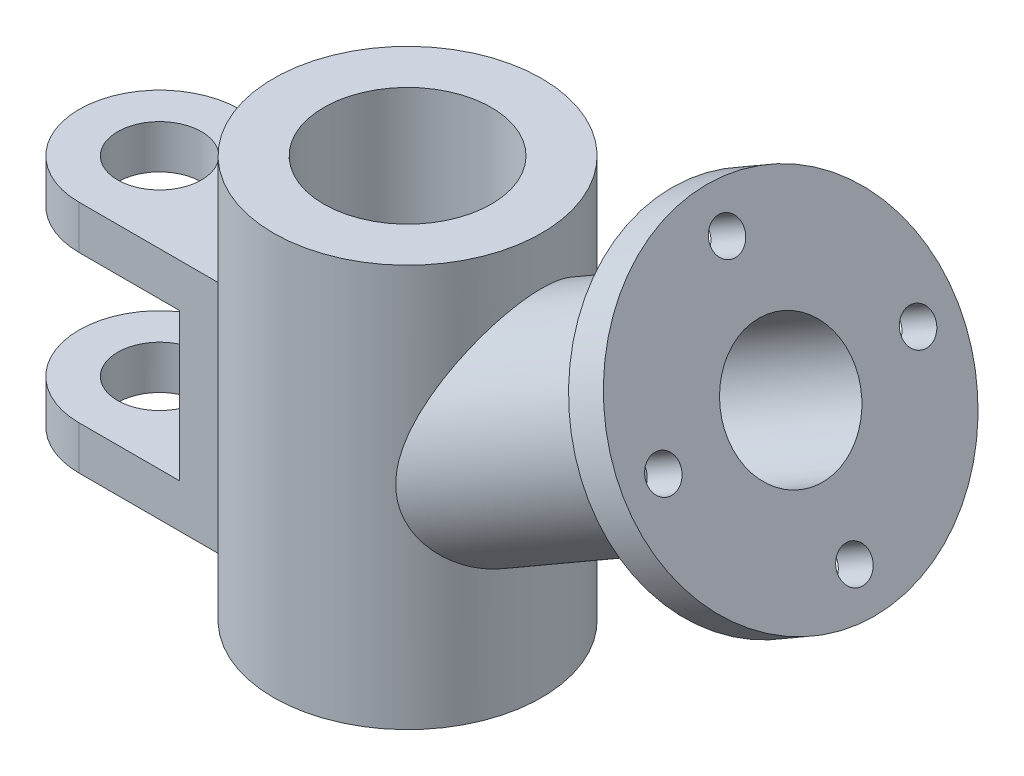
ISO-10303-21;
HEADER;
FILE_DESCRIPTION(('STEP AP214'),'2;1');
FILE_NAME('part.step','',(''),(''),'','','');
FILE_SCHEMA(('AUTOMOTIVE_DESIGN { 1 0 10303 214 1 1 1 1 }'));
ENDSEC;
DATA;
#1=APPLICATION_CONTEXT('core data for automotive mechanical design processes');
#2=APPLICATION_PROTOCOL_DEFINITION('international standard','automotive_design',2000,#1);
#3=PRODUCT_CONTEXT('',#1,'mechanical');
#4=PRODUCT('Part','Part','',(#3));
#5=PRODUCT_RELATED_PRODUCT_CATEGORY('part','',(#4));
#6=PRODUCT_DEFINITION_FORMATION('','',#4);
#7=PRODUCT_DEFINITION_CONTEXT('part definition',#1,'design');
#8=PRODUCT_DEFINITION('design','',#6,#7);
#9=PRODUCT_DEFINITION_SHAPE('','',#8);
#10=(LENGTH_UNIT() NAMED_UNIT(*) SI_UNIT(.MILLI.,.METRE.));
#11=(NAMED_UNIT(*) PLANE_ANGLE_UNIT() SI_UNIT($,.RADIAN.));
#12=(NAMED_UNIT(*) SI_UNIT($,.STERADIAN.) SOLID_ANGLE_UNIT());
#13=UNCERTAINTY_MEASURE_WITH_UNIT(LENGTH_MEASURE(1.E-05),#10,'distance_accuracy_value','');
#14=(GEOMETRIC_REPRESENTATION_CONTEXT(3) GLOBAL_UNCERTAINTY_ASSIGNED_CONTEXT((#13)) GLOBAL_UNIT_ASSIGNED_CONTEXT((#10,
#11,#12)) REPRESENTATION_CONTEXT('',''));
#15=CARTESIAN_POINT('',(0.,0.,0.));
#16=DIRECTION('',(0.,0.,1.));
#17=DIRECTION('',(1.,0.,0.));
#18=AXIS2_PLACEMENT_3D('',#15,#16,#17);
#19=CARTESIAN_POINT('',(-3.7,0.65,0.));
#20=DIRECTION('',(0.,1.,0.));
#21=DIRECTION('',(0.,0.,1.));
#22=AXIS2_PLACEMENT_3D('',#19,#20,#21);
#23=CYLINDRICAL_SURFACE('',#22,1.2);
#24=CARTESIAN_POINT('',(-3.7,3.5,0.));
#25=DIRECTION('',(0.,1.,0.));
#26=DIRECTION('',(0.,0.,1.));
#27=AXIS2_PLACEMENT_3D('',#24,#25,#26);
#28=CIRCLE('',#27,1.2);
#29=CARTESIAN_POINT('',(-3.7,3.5,1.2));
#30=VERTEX_POINT('',#29);
#31=CARTESIAN_POINT('',(-3.7,3.5,-1.2));
#32=VERTEX_POINT('',#31);
#33=EDGE_CURVE('E138',#30,#32,#28,.F.);
#34=ORIENTED_EDGE('',*,*,#33,.F.);
#35=DIRECTION('',(0.,1.,0.));
#36=VECTOR('',#35,1.);
#37=CARTESIAN_POINT('',(-3.7,0.65,1.2));
#38=LINE('',#37,#36);
#39=CARTESIAN_POINT('',(-3.7,4.15,1.2));
#40=VERTEX_POINT('',#39);
#41=EDGE_CURVE('E161',#30,#40,#38,.T.);
#42=ORIENTED_EDGE('',*,*,#41,.T.);
#43=CARTESIAN_POINT('',(-3.7,4.15,0.));
#44=DIRECTION('',(0.,1.,0.));
#45=DIRECTION('',(0.,0.,1.));
#46=AXIS2_PLACEMENT_3D('',#43,#44,#45);
#47=CIRCLE('',#46,1.2);
#48=CARTESIAN_POINT('',(-3.7,4.15,-1.2));
#49=VERTEX_POINT('',#48);
#50=EDGE_CURVE('E149',#49,#40,#47,.T.);
#51=ORIENTED_EDGE('',*,*,#50,.F.);
#52=DIRECTION('',(0.,1.,0.));
#53=VECTOR('',#52,1.);
#54=CARTESIAN_POINT('',(-3.7,0.65,-1.2));
#55=LINE('',#54,#53);
#56=EDGE_CURVE('E168',#32,#49,#55,.T.);
#57=ORIENTED_EDGE('',*,*,#56,.F.);
#58=EDGE_LOOP('',(#34,#42,#51,#57));
#59=FACE_BOUND('',#58,.T.);
#60=ADVANCED_FACE('F37',(#59),#23,.T.);
#61=CARTESIAN_POINT('',(-3.7,0.65,0.));
#62=DIRECTION('',(0.,1.,0.));
#63=DIRECTION('',(0.,0.,1.));
#64=AXIS2_PLACEMENT_3D('',#61,#62,#63);
#65=CYLINDRICAL_SURFACE('',#64,0.625);
#66=CARTESIAN_POINT('',(-3.7,3.5,0.));
#67=DIRECTION('',(0.,1.,0.));
#68=DIRECTION('',(0.,0.,1.));
#69=AXIS2_PLACEMENT_3D('',#66,#67,#68);
#70=CIRCLE('',#69,0.625);
#71=CARTESIAN_POINT('',(-3.7,3.5,0.625));
#72=VERTEX_POINT('',#71);
#73=EDGE_CURVE('E44',#72,#72,#70,.F.);
#74=ORIENTED_EDGE('',*,*,#73,.T.);
#75=EDGE_LOOP('',(#74));
#76=FACE_BOUND('',#75,.T.);
#77=CARTESIAN_POINT('',(-3.7,4.15,0.));
#78=DIRECTION('',(0.,1.,0.));
#79=DIRECTION('',(0.,0.,1.));
#80=AXIS2_PLACEMENT_3D('',#77,#78,#79);
#81=CIRCLE('',#80,0.625);
#82=CARTESIAN_POINT('',(-3.7,4.15,0.625));
#83=VERTEX_POINT('',#82);
#84=EDGE_CURVE('E144',#83,#83,#81,.T.);
#85=ORIENTED_EDGE('',*,*,#84,.T.);
#86=EDGE_LOOP('',(#85));
#87=FACE_BOUND('',#86,.T.);
#88=ADVANCED_FACE('F207',(#76,#87),#65,.F.);
#89=CARTESIAN_POINT('',(0.,6.,0.));
#90=DIRECTION('',(0.,-1.,0.));
#91=DIRECTION('',(0.,0.,-1.));
#92=AXIS2_PLACEMENT_3D('',#89,#90,#91);
#93=CYLINDRICAL_SURFACE('',#92,2.);
#94=CARTESIAN_POINT('',(2.,5.28675134594813,0.));
#95=CARTESIAN_POINT('',(1.9999970486525,5.28674553568537,-0.0509645549548926));
#96=CARTESIAN_POINT('',(1.99803036507296,5.28258531444875,-0.101968074915427));
#97=CARTESIAN_POINT('',(1.99037092425183,5.26634323343092,-0.202425088211594));
#98=CARTESIAN_POINT('',(1.98467255223197,5.25424943657451,-0.251876127969954));
#99=CARTESIAN_POINT('',(1.96845268767769,5.21968619808088,-0.358794338921624));
#100=CARTESIAN_POINT('',(1.95713760119165,5.195501316032,-0.415581233530213));
#101=CARTESIAN_POINT('',(1.93093069375908,5.13907333325674,-0.524059647410448));
#102=CARTESIAN_POINT('',(1.91603305556804,5.10681712305062,-0.575742684638304));
#103=CARTESIAN_POINT('',(1.87551765385294,5.01824597695864,-0.698951661092725));
#104=CARTESIAN_POINT('',(1.84830951140444,4.95805490178913,-0.767139974964058));
#105=CARTESIAN_POINT('',(1.7909867316854,4.8285693881339,-0.892836810800664));
#106=CARTESIAN_POINT('',(1.76086375165627,4.75924860140653,-0.950313212267064));
#107=CARTESIAN_POINT('',(1.70535745654534,4.62776578435047,-1.04604468652679));
#108=CARTESIAN_POINT('',(1.68013462820626,4.56667024504012,-1.08588649630983));
#109=CARTESIAN_POINT('',(1.62986640225519,4.44105499584961,-1.15997484965928));
#110=CARTESIAN_POINT('',(1.60482115283824,4.37653273775444,-1.19421714983622));
#111=CARTESIAN_POINT('',(1.55573541972518,4.24458477197344,-1.25749289608485));
#112=CARTESIAN_POINT('',(1.53169539806281,4.17715775746073,-1.28652396666901));
#113=CARTESIAN_POINT('',(1.48557417432718,4.03974300659564,-1.33951570213413));
#114=CARTESIAN_POINT('',(1.46349179029028,3.96975685193415,-1.3634794387979));
#115=CARTESIAN_POINT('',(1.41737118784856,3.80982531233715,-1.41153033550627));
#116=CARTESIAN_POINT('',(1.39418361541946,3.71919784518041,-1.43420363642414));
#117=CARTESIAN_POINT('',(1.35581738360888,3.53454566238734,-1.47053291818328));
#118=CARTESIAN_POINT('',(1.3406189505389,3.44052995573783,-1.48421118366653));
#119=CARTESIAN_POINT('',(1.32526567903617,3.27709274870488,-1.49791385075284));
#120=CARTESIAN_POINT('',(1.32207565854465,3.20821891129919,-1.50070229442481));
#121=CARTESIAN_POINT('',(1.32401342684527,3.07068145547059,-1.49899977723801));
#122=CARTESIAN_POINT('',(1.32912553603763,3.0020176855799,-1.49452253853183));
#123=CARTESIAN_POINT('',(1.34876732528906,2.86641719439632,-1.47682225044538));
#124=CARTESIAN_POINT('',(1.3633893615177,2.79950417591694,-1.46351340644034));
#125=CARTESIAN_POINT('',(1.40117326229666,2.67083315424934,-1.42736768376759));
#126=CARTESIAN_POINT('',(1.42433998211984,2.60907810644702,-1.40452538701438));
#127=CARTESIAN_POINT('',(1.47309929261382,2.49984301956458,-1.3531675444883));
#128=CARTESIAN_POINT('',(1.4980229287275,2.45154406885291,-1.32572324583763));
#129=CARTESIAN_POINT('',(1.55008786188708,2.36053090509224,-1.26445447180689));
#130=CARTESIAN_POINT('',(1.57723009683264,2.31781907401334,-1.23062729011099));
#131=CARTESIAN_POINT('',(1.6362694232045,2.23143378908336,-1.15127823856732));
#132=CARTESIAN_POINT('',(1.66822410068182,2.18872669231969,-1.10474952104184));
#133=CARTESIAN_POINT('',(1.73021780268166,2.11046463930542,-1.00489325473654));
#134=CARTESIAN_POINT('',(1.7602556711338,2.07491397192563,-0.951561660059982));
#135=CARTESIAN_POINT('',(1.8215574324917,2.00511658459749,-0.829094013256131));
#136=CARTESIAN_POINT('',(1.85210385038894,1.97220471861288,-0.758829269900914));
#137=CARTESIAN_POINT('',(1.90571090628462,1.91599178606554,-0.611874293037778));
#138=CARTESIAN_POINT('',(1.92877005697721,1.89269262876782,-0.535182786689392));
#139=CARTESIAN_POINT('',(1.96612928486342,1.85547486260921,-0.375729769907822));
#140=CARTESIAN_POINT('',(1.98023968653309,1.84175879794579,-0.292875926358499));
#141=CARTESIAN_POINT('',(1.99787194717028,1.82467517260186,-0.125009022886388));
#142=CARTESIAN_POINT('',(2.0013960858517,1.82130538388436,-0.0399964318192956));
#143=CARTESIAN_POINT('',(1.99767178786206,1.82489112866947,0.126401053537316));
#144=CARTESIAN_POINT('',(1.99081819833639,1.83146819713097,0.207803514204965));
#145=CARTESIAN_POINT('',(1.96754322783607,1.85416242103331,0.367848133815773));
#146=CARTESIAN_POINT('',(1.9511225356101,1.87027888972115,0.446490491030453));
#147=CARTESIAN_POINT('',(1.90980367359583,1.91193169591238,0.599094917937578));
#148=CARTESIAN_POINT('',(1.88488577831092,1.93748996331462,0.673045618295913));
#149=CARTESIAN_POINT('',(1.82830377070922,1.99793792859396,0.814308871040709));
#150=CARTESIAN_POINT('',(1.79663459209368,2.03283463927503,0.881616382441848));
#151=CARTESIAN_POINT('',(1.72755963362521,2.11362673862452,1.01048900698373));
#152=CARTESIAN_POINT('',(1.68997619906204,2.15990332800566,1.07172066544373));
#153=CARTESIAN_POINT('',(1.6136025499884,2.26308586171886,1.18357698326777));
#154=CARTESIAN_POINT('',(1.57481371861604,2.3199799728611,1.23421331909035));
#155=CARTESIAN_POINT('',(1.50996145383683,2.4294114009334,1.31222586871969));
#156=CARTESIAN_POINT('',(1.48311287682947,2.47958507915393,1.34226029031302));
#157=CARTESIAN_POINT('',(1.43403484798806,2.58582820557518,1.39457166425866));
#158=CARTESIAN_POINT('',(1.41179654291347,2.64188603634136,1.41686354153033));
#159=CARTESIAN_POINT('',(1.37412739986106,2.75901498960152,1.45343747366988));
#160=CARTESIAN_POINT('',(1.35872528529978,2.82010600995811,1.46768579904074));
#161=CARTESIAN_POINT('',(1.33602066041981,2.94505045755975,1.48838326101344));
#162=CARTESIAN_POINT('',(1.32872485917987,3.00890612758975,1.49482593777565));
#163=CARTESIAN_POINT('',(1.32090236801746,3.15447738653167,1.50175223890729));
#164=CARTESIAN_POINT('',(1.32271103592767,3.23639731724767,1.50017854643198));
#165=CARTESIAN_POINT('',(1.33580137367746,3.39891425648451,1.48851876488665));
#166=CARTESIAN_POINT('',(1.34711435679016,3.47950599305465,1.47840453728718));
#167=CARTESIAN_POINT('',(1.37422073426935,3.62717221607955,1.45320652203402));
#168=CARTESIAN_POINT('',(1.38917140172567,3.69456688661104,1.43901031981333));
#169=CARTESIAN_POINT('',(1.4224713427755,3.82742285900561,1.40610216953895));
#170=CARTESIAN_POINT('',(1.44082329660041,3.89288258862779,1.3873866566974));
#171=CARTESIAN_POINT('',(1.47986276585991,4.02185197422553,1.34566894680336));
#172=CARTESIAN_POINT('',(1.50055502122334,4.08535732882995,1.32265798640131));
#173=CARTESIAN_POINT('',(1.54339714295202,4.21013132612929,1.27240563982987));
#174=CARTESIAN_POINT('',(1.56554640368221,4.27140088192046,1.24516600507478));
#175=CARTESIAN_POINT('',(1.60805791263721,4.38466557044923,1.18963445102772));
#176=CARTESIAN_POINT('',(1.62833707302591,4.43692322817819,1.16181417124925));
#177=CARTESIAN_POINT('',(1.66906630346155,4.53923869329852,1.10250271783841));
#178=CARTESIAN_POINT('',(1.689516337527,4.58929695059075,1.0710122998146));
#179=CARTESIAN_POINT('',(1.73008318094181,4.68665211306674,1.00415977583565));
#180=CARTESIAN_POINT('',(1.7502008577014,4.73395746917606,0.96881059430578));
#181=CARTESIAN_POINT('',(1.78966516512206,4.82533331714667,0.893808138305228));
#182=CARTESIAN_POINT('',(1.80901237163407,4.86940624648568,0.854158164049344));
#183=CARTESIAN_POINT('',(1.84806600077724,4.95730774131388,0.766272620041581));
#184=CARTESIAN_POINT('',(1.86764400675991,5.0007467728831,0.717583720445762));
#185=CARTESIAN_POINT('',(1.904180363692,5.08103454011871,0.61408475785194));
#186=CARTESIAN_POINT('',(1.92114051683689,5.11788781236879,0.559278951076864));
#187=CARTESIAN_POINT('',(1.94844910343736,5.17684036449463,0.453829768030057));
#188=CARTESIAN_POINT('',(1.95943689871934,5.2003977446446,0.404177738052494));
#189=CARTESIAN_POINT('',(1.97785973227975,5.23975954934716,0.301297519571608));
#190=CARTESIAN_POINT('',(1.98530333001162,5.25558265512881,0.248078304654108));
#191=CARTESIAN_POINT('',(1.99368655715187,5.27337683667634,0.161978994939816));
#192=CARTESIAN_POINT('',(1.99604359010548,5.2783718790058,0.129841001902964));
#193=CARTESIAN_POINT('',(1.99920135148534,5.28506119569592,0.0651406813479076));
#194=CARTESIAN_POINT('',(2.00000188660314,5.28675506006852,0.0325783016287044));
#195=CARTESIAN_POINT('',(2.,5.28675134594813,0.));
#196=B_SPLINE_CURVE_WITH_KNOTS('',3,(#94,#95,#96,#97,#98,#99,#100,#101,#102,#103,#104,#105,#106,
#107,#108,#109,#110,#111,#112,#113,#114,#115,#116,#117,#118,#119,#120,#121,#122,#123,#124,#125,
#126,#127,#128,#129,#130,#131,#132,#133,#134,#135,#136,#137,#138,#139,#140,#141,#142,#143,#144,
#145,#146,#147,#148,#149,#150,#151,#152,#153,#154,#155,#156,#157,#158,#159,#160,#161,#162,#163,
#164,#165,#166,#167,#168,#169,#170,#171,#172,#173,#174,#175,#176,#177,#178,#179,#180,#181,#182,
#183,#184,#185,#186,#187,#188,#189,#190,#191,#192,#193,#194,#195),.UNSPECIFIED.,.T.,.F.,(4,2,2,
2,2,2,2,2,2,2,2,2,2,2,2,2,2,2,2,2,2,2,2,2,2,2,2,2,2,2,2,2,2,2,2,2,2,2,2,2,2,2,2,2,2,2,2,2,2,2,
4),(0.,0.15276354826251,0.305757477570657,0.4929639085865,0.680476397337383,0.963704315388515,
1.24776831048418,1.47899948637416,1.71040508858541,1.94191590835847,2.17328598298484,
2.46145461217104,2.74890660464451,2.95522920350617,3.16116258955364,3.36912638856181,
3.57720853957934,3.75918582207613,3.94124043626816,4.1528050091894,4.36449599840936,
4.61350800514627,4.86256944657616,5.11674752585729,5.3708708648723,5.61556537554982,
5.86024227251474,6.10549107591859,6.35092457089976,6.60608846141651,6.8609696528724,
7.05323202781902,7.2451217039618,7.43781017644694,7.63065800638002,7.87513888882805,
8.12042842035551,8.33157859806514,8.54289587616731,8.75464908036291,8.96631481436553,
9.15391855925452,9.34148374826157,9.52843894448834,9.7152516821129,9.91911693538211,
10.1228412106648,10.2903584771779,10.4574691010694,10.5551087054079,10.6527604352733),.UNSPECIFIED.);
#197=CARTESIAN_POINT('',(2.,5.28675134594813,0.));
#198=VERTEX_POINT('',#197);
#199=EDGE_CURVE('E130',#198,#198,#196,.T.);
#200=ORIENTED_EDGE('',*,*,#199,.T.);
#201=EDGE_LOOP('',(#200));
#202=FACE_BOUND('',#201,.T.);
#203=CARTESIAN_POINT('',(0.,0.,0.));
#204=DIRECTION('',(0.,1.,0.));
#205=DIRECTION('',(0.,0.,1.));
#206=AXIS2_PLACEMENT_3D('',#203,#204,#205);
#207=CIRCLE('',#206,2.);
#208=CARTESIAN_POINT('',(0.,0.,2.));
#209=VERTEX_POINT('',#208);
#210=EDGE_CURVE('E177',#209,#209,#207,.T.);
#211=ORIENTED_EDGE('',*,*,#210,.T.);
#212=EDGE_LOOP('',(#211));
#213=FACE_BOUND('',#212,.T.);
#214=CARTESIAN_POINT('',(0.,6.,0.));
#215=DIRECTION('',(0.,1.,0.));
#216=DIRECTION('',(0.,0.,1.));
#217=AXIS2_PLACEMENT_3D('',#214,#215,#216);
#218=CIRCLE('',#217,2.);
#219=CARTESIAN_POINT('',(0.,6.,2.));
#220=VERTEX_POINT('',#219);
#221=EDGE_CURVE('E176',#220,#220,#218,.T.);
#222=ORIENTED_EDGE('',*,*,#221,.F.);
#223=EDGE_LOOP('',(#222));
#224=FACE_BOUND('',#223,.T.);
#225=CARTESIAN_POINT('',(0.,0.65,0.));
#226=DIRECTION('',(0.,1.,0.));
#227=DIRECTION('',(0.,0.,1.));
#228=AXIS2_PLACEMENT_3D('',#225,#226,#227);
#229=CIRCLE('',#228,2.);
#230=CARTESIAN_POINT('',(-1.6,0.65,-1.2));
#231=VERTEX_POINT('',#230);
#232=CARTESIAN_POINT('',(-1.6,0.65,1.2));
#233=VERTEX_POINT('',#232);
#234=EDGE_CURVE('E12',#231,#233,#229,.T.);
#235=ORIENTED_EDGE('',*,*,#234,.F.);
#236=DIRECTION('',(0.,-1.,0.));
#237=VECTOR('',#236,1.);
#238=CARTESIAN_POINT('',(-1.6,6.,-1.2));
#239=LINE('',#238,#237);
#240=CARTESIAN_POINT('',(-1.6,4.15,-1.2));
#241=VERTEX_POINT('',#240);
#242=EDGE_CURVE('E49',#231,#241,#239,.F.);
#243=ORIENTED_EDGE('',*,*,#242,.T.);
#244=CARTESIAN_POINT('',(0.,4.15,0.));
#245=DIRECTION('',(0.,1.,0.));
#246=DIRECTION('',(0.,0.,1.));
#247=AXIS2_PLACEMENT_3D('',#244,#245,#246);
#248=CIRCLE('',#247,2.);
#249=CARTESIAN_POINT('',(-1.6,4.15,1.2));
#250=VERTEX_POINT('',#249);
#251=EDGE_CURVE('E185',#241,#250,#248,.T.);
#252=ORIENTED_EDGE('',*,*,#251,.T.);
#253=DIRECTION('',(0.,-1.,0.));
#254=VECTOR('',#253,1.);
#255=CARTESIAN_POINT('',(-1.6,6.,1.2));
#256=LINE('',#255,#254);
#257=EDGE_CURVE('E190',#250,#233,#256,.T.);
#258=ORIENTED_EDGE('',*,*,#257,.T.);
#259=EDGE_LOOP('',(#235,#243,#252,#258));
#260=FACE_BOUND('',#259,.T.);
#261=ADVANCED_FACE('F45',(#202,#213,#224,#260),#93,.T.);
#262=CARTESIAN_POINT('',(0.,6.,0.));
#263=DIRECTION('',(0.,1.,0.));
#264=DIRECTION('',(0.,0.,1.));
#265=AXIS2_PLACEMENT_3D('',#262,#263,#264);
#266=PLANE('',#265);
#267=ORIENTED_EDGE('',*,*,#221,.T.);
#268=EDGE_LOOP('',(#267));
#269=FACE_BOUND('',#268,.T.);
#270=CARTESIAN_POINT('',(0.,6.,0.));
#271=DIRECTION('',(0.,1.,0.));
#272=DIRECTION('',(0.,0.,1.));
#273=AXIS2_PLACEMENT_3D('',#270,#271,#272);
#274=CIRCLE('',#273,1.25);
#275=CARTESIAN_POINT('',(0.,6.,1.25));
#276=VERTEX_POINT('',#275);
#277=EDGE_CURVE('E173',#276,#276,#274,.T.);
#278=ORIENTED_EDGE('',*,*,#277,.F.);
#279=EDGE_LOOP('',(#278));
#280=FACE_BOUND('',#279,.T.);
#281=ADVANCED_FACE('F390',(#269,#280),#266,.T.);
#282=CARTESIAN_POINT('',(0.,0.,0.));
#283=DIRECTION('',(0.,1.,0.));
#284=DIRECTION('',(0.,0.,1.));
#285=AXIS2_PLACEMENT_3D('',#282,#283,#284);
#286=PLANE('',#285);
#287=ORIENTED_EDGE('',*,*,#210,.F.);
#288=EDGE_LOOP('',(#287));
#289=FACE_BOUND('',#288,.T.);
#290=CARTESIAN_POINT('',(0.,0.,0.));
#291=DIRECTION('',(0.,1.,0.));
#292=DIRECTION('',(0.,0.,1.));
#293=AXIS2_PLACEMENT_3D('',#290,#291,#292);
#294=CIRCLE('',#293,1.25);
#295=CARTESIAN_POINT('',(0.,0.,1.25));
#296=VERTEX_POINT('',#295);
#297=EDGE_CURVE('E166',#296,#296,#294,.T.);
#298=ORIENTED_EDGE('',*,*,#297,.T.);
#299=EDGE_LOOP('',(#298));
#300=FACE_BOUND('',#299,.T.);
#301=ADVANCED_FACE('F252',(#289,#300),#286,.F.);
#302=CARTESIAN_POINT('',(0.,6.,0.));
#303=DIRECTION('',(0.,-1.,0.));
#304=DIRECTION('',(0.,0.,-1.));
#305=AXIS2_PLACEMENT_3D('',#302,#303,#304);
#306=CYLINDRICAL_SURFACE('',#305,1.25);
#307=CARTESIAN_POINT('',(1.25,4.21865334794732,0.));
#308=CARTESIAN_POINT('',(1.24999813614527,4.21864970328222,0.0321026990287067));
#309=CARTESIAN_POINT('',(1.24874910116528,4.21603274633786,0.0642414788663816));
#310=CARTESIAN_POINT('',(1.24388323854935,4.2058141021631,0.127550186545698));
#311=CARTESIAN_POINT('',(1.24026178878809,4.19820268428277,0.158718098435612));
#312=CARTESIAN_POINT('',(1.22995121638852,4.17644874622317,0.226112293741986));
#313=CARTESIAN_POINT('',(1.22275692816389,4.16122578138426,0.261909514552392));
#314=CARTESIAN_POINT('',(1.20609104993659,4.12571330757059,0.330287681274534));
#315=CARTESIAN_POINT('',(1.19661595820644,4.10541600607837,0.36286357190049));
#316=CARTESIAN_POINT('',(1.17081220210405,4.04963137184636,0.44060789765104));
#317=CARTESIAN_POINT('',(1.15346152015805,4.01169379212786,0.483661057654697));
#318=CARTESIAN_POINT('',(1.11687776017897,3.93009437997939,0.563028763773868));
#319=CARTESIAN_POINT('',(1.09763924768612,3.88641589107644,0.599322929048331));
#320=CARTESIAN_POINT('',(1.06202138702507,3.80328761309725,0.660008718693008));
#321=CARTESIAN_POINT('',(1.04574846626571,3.76448547529165,0.685367503879216));
#322=CARTESIAN_POINT('',(1.01328078247239,3.68470717725178,0.73251773677677));
#323=CARTESIAN_POINT('',(0.997086089141574,3.64372936861845,0.754306427024871));
#324=CARTESIAN_POINT('',(0.96530170805266,3.55993319466213,0.794575147664763));
#325=CARTESIAN_POINT('',(0.949712312840895,3.51711395992198,0.813053593398418));
#326=CARTESIAN_POINT('',(0.919747236941378,3.42985128837338,0.846802122620772));
#327=CARTESIAN_POINT('',(0.905370820003192,3.38540886062635,0.862074160828975));
#328=CARTESIAN_POINT('',(0.875416784742906,3.28435933544799,0.892580979692902));
#329=CARTESIAN_POINT('',(0.860345772020769,3.22733996310972,0.906970167297517));
#330=CARTESIAN_POINT('',(0.8351863624843,3.11113441698942,0.93019361500459));
#331=CARTESIAN_POINT('',(0.825086038946662,3.0519537994329,0.939041185782719));
#332=CARTESIAN_POINT('',(0.814544566679323,2.94920919789628,0.948183324565382));
#333=CARTESIAN_POINT('',(0.812167597853762,2.90601707007576,0.950199871613304));
#334=CARTESIAN_POINT('',(0.812675545600198,2.81968887356437,0.949769797426733));
#335=CARTESIAN_POINT('',(0.815550126862748,2.77655286159755,0.947331942673071));
#336=CARTESIAN_POINT('',(0.82734512093803,2.69124838948537,0.93704997913504));
#337=CARTESIAN_POINT('',(0.836328630735141,2.649094823313,0.929149433690343));
#338=CARTESIAN_POINT('',(0.859864631634575,2.56797914574299,0.90740397109388));
#339=CARTESIAN_POINT('',(0.874420070179208,2.52901873672928,0.893555907346669));
#340=CARTESIAN_POINT('',(0.905111669361618,2.46033806665069,0.862370457122187));
#341=CARTESIAN_POINT('',(0.920782355246301,2.43007758269728,0.845739171229618));
#342=CARTESIAN_POINT('',(0.953614681067882,2.37299267998655,0.808538843689019));
#343=CARTESIAN_POINT('',(0.970776995531826,2.3461698294662,0.78796801543309));
#344=CARTESIAN_POINT('',(1.00829540200622,2.29171534591807,0.739544311274648));
#345=CARTESIAN_POINT('',(1.02870685844176,2.26469464124826,0.711049139016081));
#346=CARTESIAN_POINT('',(1.06845670494612,2.215049199112,0.649798021166723));
#347=CARTESIAN_POINT('',(1.08779443421615,2.19242714772653,0.61703949236814));
#348=CARTESIAN_POINT('',(1.12768984115862,2.14757049962821,0.541270698358137));
#349=CARTESIAN_POINT('',(1.14778891732761,2.1262148780489,0.497492467310776));
#350=CARTESIAN_POINT('',(1.18334617794659,2.08948842484067,0.405729083119038));
#351=CARTESIAN_POINT('',(1.19880327000102,2.07411900168825,0.357742943157027));
#352=CARTESIAN_POINT('',(1.22429963303666,2.04915051114397,0.257540600515593));
#353=CARTESIAN_POINT('',(1.23419394696004,2.03970515099553,0.205248681744495));
#354=CARTESIAN_POINT('',(1.24721384243214,2.02733104087638,0.0990790745609366));
#355=CARTESIAN_POINT('',(1.25034104142277,2.02440073370576,0.0452017682010726));
#356=CARTESIAN_POINT('',(1.2496143115555,2.02508596093283,-0.0602937224010105));
#357=CARTESIAN_POINT('',(1.24603531526447,2.02844370225563,-0.111915856706425));
#358=CARTESIAN_POINT('',(1.232683544034,2.04114977187746,-0.213588085827169));
#359=CARTESIAN_POINT('',(1.22291128000496,2.05049760602761,-0.263638309958985));
#360=CARTESIAN_POINT('',(1.19785923536017,2.07505707692805,-0.36075748893584));
#361=CARTESIAN_POINT('',(1.18258597468951,2.09026177342694,-0.407829895855065));
#362=CARTESIAN_POINT('',(1.14756162561547,2.12646188721477,-0.497936167775832));
#363=CARTESIAN_POINT('',(1.12780755766145,2.14746115967683,-0.540967318464282));
#364=CARTESIAN_POINT('',(1.08433851370691,2.19628936935301,-0.623684272381126));
#365=CARTESIAN_POINT('',(1.060492136477,2.22436786610046,-0.663153998685726));
#366=CARTESIAN_POINT('',(1.01159163893849,2.28712426611613,-0.735584303583659));
#367=CARTESIAN_POINT('',(0.986538488008199,2.32179693630893,-0.768550001731208));
#368=CARTESIAN_POINT('',(0.943955310189886,2.38895120001299,-0.819930890727398));
#369=CARTESIAN_POINT('',(0.926057832556045,2.41997749096286,-0.839940750394299));
#370=CARTESIAN_POINT('',(0.892938000205868,2.48594213279277,-0.875067752063272));
#371=CARTESIAN_POINT('',(0.87771030035859,2.52087243235558,-0.890194722350042));
#372=CARTESIAN_POINT('',(0.851464812509628,2.59429182913414,-0.915339413392153));
#373=CARTESIAN_POINT('',(0.840472512843486,2.63280079316032,-0.925326318720514));
#374=CARTESIAN_POINT('',(0.823830943115782,2.71190260756079,-0.94017468856974));
#375=CARTESIAN_POINT('',(0.818184786166763,2.7524966576163,-0.945033166944918));
#376=CARTESIAN_POINT('',(0.811522963885866,2.84235194078356,-0.950765885076619));
#377=CARTESIAN_POINT('',(0.811635383410467,2.89174865366688,-0.950669468190259));
#378=CARTESIAN_POINT('',(0.81775058885594,2.98992103952507,-0.945405769130707));
#379=CARTESIAN_POINT('',(0.823770583414345,3.03869447638518,-0.940223672479935));
#380=CARTESIAN_POINT('',(0.838838295322252,3.1283070211887,-0.926788438465457));
#381=CARTESIAN_POINT('',(0.847360700322198,3.16932056492162,-0.919050919896149));
#382=CARTESIAN_POINT('',(0.866607232338006,3.25025099593715,-0.900925435149091));
#383=CARTESIAN_POINT('',(0.877333095701186,3.29016699004074,-0.890535377166827));
#384=CARTESIAN_POINT('',(0.900345417394656,3.36895537952556,-0.86726413042715));
#385=CARTESIAN_POINT('',(0.912637111777876,3.40782371742477,-0.854374504030582));
#386=CARTESIAN_POINT('',(0.938238760963884,3.48433031892558,-0.826178531887488));
#387=CARTESIAN_POINT('',(0.951548822612531,3.52196845286277,-0.810871932375353));
#388=CARTESIAN_POINT('',(0.980003250046636,3.59925237596733,-0.77629863425639));
#389=CARTESIAN_POINT('',(0.99520483527315,3.63877350686977,-0.756799389533526));
#390=CARTESIAN_POINT('',(1.02587974134444,3.71604011224703,-0.714668291611172));
#391=CARTESIAN_POINT('',(1.04135320571359,3.75378460765153,-0.692034737618168));
#392=CARTESIAN_POINT('',(1.07203128336141,3.82688867503852,-0.643482398054762));
#393=CARTESIAN_POINT('',(1.08723692135612,3.86226050984017,-0.617582883726999));
#394=CARTESIAN_POINT('',(1.11695931946486,3.93020916190778,-0.562043724284678));
#395=CARTESIAN_POINT('',(1.1314769913262,3.96278972746879,-0.532409231295577));
#396=CARTESIAN_POINT('',(1.15735686405484,4.02012517277403,-0.473205665808765));
#397=CARTESIAN_POINT('',(1.16888106921439,4.0453434929776,-0.444161540350015));
#398=CARTESIAN_POINT('',(1.19043404703174,4.09211118344551,-0.38265898759457));
#399=CARTESIAN_POINT('',(1.20046176467966,4.11365796681372,-0.350198178804163));
#400=CARTESIAN_POINT('',(1.21843869037146,4.15205875918627,-0.281403604004611));
#401=CARTESIAN_POINT('',(1.22635786243426,4.16884515531613,-0.245023279758547));
#402=CARTESIAN_POINT('',(1.23905601272055,4.19567269016587,-0.169385408055287));
#403=CARTESIAN_POINT('',(1.24384793699043,4.20574164138597,-0.130140480000971));
#404=CARTESIAN_POINT('',(1.24781992704368,4.2140806369447,-0.0753111558685922));
#405=CARTESIAN_POINT('',(1.24863484074897,4.21579031802429,-0.0603162501790653));
#406=CARTESIAN_POINT('',(1.24972537085785,4.21807764668261,-0.0302169093872325));
#407=CARTESIAN_POINT('',(1.25000087741583,4.21865506368557,-0.0151124526042312));
#408=CARTESIAN_POINT('',(1.25,4.21865334794732,0.));
#409=B_SPLINE_CURVE_WITH_KNOTS('',3,(#307,#308,#309,#310,#311,#312,#313,#314,#315,#316,#317,
#318,#319,#320,#321,#322,#323,#324,#325,#326,#327,#328,#329,#330,#331,#332,#333,#334,#335,#336,
#337,#338,#339,#340,#341,#342,#343,#344,#345,#346,#347,#348,#349,#350,#351,#352,#353,#354,#355,
#356,#357,#358,#359,#360,#361,#362,#363,#364,#365,#366,#367,#368,#369,#370,#371,#372,#373,#374,
#375,#376,#377,#378,#379,#380,#381,#382,#383,#384,#385,#386,#387,#388,#389,#390,#391,#392,#393,
#394,#395,#396,#397,#398,#399,#400,#401,#402,#403,#404,#405,#406,#407,#408),.UNSPECIFIED.,.T.,
.F.,(4,2,2,2,2,2,2,2,2,2,2,2,2,2,2,2,2,2,2,2,2,2,2,2,2,2,2,2,2,2,2,2,2,2,2,2,2,2,2,2,2,2,2,2,2,
2,2,2,2,2,4),(0.,0.0962461091854084,0.192680292531519,0.310696840900612,0.428895749391761,
0.60774366668795,0.78712243985762,0.934312576875,1.0816158698249,1.22898949147428,
1.37627300730675,1.55803396407407,1.73935664916152,1.86884616013595,1.99808110385065,
2.12867156085191,2.25933119334531,2.37266665009142,2.48605362743651,2.61834744281429,
2.75072179273056,2.9080802758821,3.06547576115336,3.22680234120961,3.38809035753427,
3.54291029526456,3.69771746286691,3.85234174895706,4.00706915676485,4.16828767454405,
4.32937878066476,4.45198667616804,4.57434622482995,4.69743103335025,4.82058747139082,
4.96794742962435,5.11573792228422,5.24335937442764,5.3710817819931,5.49924308491356,
5.62741785285046,5.76714120102705,5.90694066760651,6.04595077395733,6.18477118293518,
6.30496154250676,6.42523623890345,6.54714224694145,6.66854033742829,6.71383929044772,
6.75914746724947),.UNSPECIFIED.);
#410=CARTESIAN_POINT('',(1.25,4.21865334794732,0.));
#411=VERTEX_POINT('',#410);
#412=EDGE_CURVE('E458',#411,#411,#409,.T.);
#413=ORIENTED_EDGE('',*,*,#412,.T.);
#414=EDGE_LOOP('',(#413));
#415=FACE_BOUND('',#414,.T.);
#416=ORIENTED_EDGE('',*,*,#277,.T.);
#417=EDGE_LOOP('',(#416));
#418=FACE_BOUND('',#417,.T.);
#419=ORIENTED_EDGE('',*,*,#297,.F.);
#420=EDGE_LOOP('',(#419));
#421=FACE_BOUND('',#420,.T.);
#422=ADVANCED_FACE('F250',(#415,#418,#421),#306,.F.);
#423=CARTESIAN_POINT('',(-3.7,0.65,-1.2));
#424=DIRECTION('',(0.,0.,-1.));
#425=DIRECTION('',(-1.,0.,0.));
#426=AXIS2_PLACEMENT_3D('',#423,#424,#425);
#427=PLANE('',#426);
#428=DIRECTION('',(1.,0.,0.));
#429=VECTOR('',#428,1.);
#430=CARTESIAN_POINT('',(-3.7,3.5,-1.2));
#431=LINE('',#430,#429);
#432=CARTESIAN_POINT('',(-2.2,3.5,-1.2));
#433=VERTEX_POINT('',#432);
#434=EDGE_CURVE('E142',#32,#433,#431,.T.);
#435=ORIENTED_EDGE('',*,*,#434,.F.);
#436=ORIENTED_EDGE('',*,*,#56,.T.);
#437=DIRECTION('',(-1.,0.,0.));
#438=VECTOR('',#437,1.);
#439=CARTESIAN_POINT('',(-3.7,4.15,-1.2));
#440=LINE('',#439,#438);
#441=EDGE_CURVE('E156',#241,#49,#440,.T.);
#442=ORIENTED_EDGE('',*,*,#441,.F.);
#443=ORIENTED_EDGE('',*,*,#242,.F.);
#444=DIRECTION('',(-1.,0.,0.));
#445=VECTOR('',#444,1.);
#446=CARTESIAN_POINT('',(-3.7,0.65,-1.2));
#447=LINE('',#446,#445);
#448=CARTESIAN_POINT('',(-3.7,0.65,-1.2));
#449=VERTEX_POINT('',#448);
#450=EDGE_CURVE('E157',#231,#449,#447,.T.);
#451=ORIENTED_EDGE('',*,*,#450,.T.);
#452=CARTESIAN_POINT('',(-3.7,1.3,-1.2));
#453=VERTEX_POINT('',#452);
#454=EDGE_CURVE('E167',#449,#453,#55,.T.);
#455=ORIENTED_EDGE('',*,*,#454,.T.);
#456=DIRECTION('',(-1.,0.,0.));
#457=VECTOR('',#456,1.);
#458=CARTESIAN_POINT('',(-3.7,1.3,-1.2));
#459=LINE('',#458,#457);
#460=CARTESIAN_POINT('',(-2.2,1.3,-1.2));
#461=VERTEX_POINT('',#460);
#462=EDGE_CURVE('E59',#461,#453,#459,.T.);
#463=ORIENTED_EDGE('',*,*,#462,.F.);
#464=DIRECTION('',(0.,-1.,0.));
#465=VECTOR('',#464,1.);
#466=CARTESIAN_POINT('',(-2.2,0.65,-1.2));
#467=LINE('',#466,#465);
#468=EDGE_CURVE('E117',#433,#461,#467,.T.);
#469=ORIENTED_EDGE('',*,*,#468,.F.);
#470=EDGE_LOOP('',(#435,#436,#442,#443,#451,#455,#463,#469));
#471=FACE_BOUND('',#470,.T.);
#472=ADVANCED_FACE('F232',(#471),#427,.T.);
#473=CARTESIAN_POINT('',(-1.46144263171015,0.65,1.2));
#474=DIRECTION('',(0.,0.,1.));
#475=DIRECTION('',(1.,0.,0.));
#476=AXIS2_PLACEMENT_3D('',#473,#474,#475);
#477=PLANE('',#476);
#478=DIRECTION('',(-1.,0.,0.));
#479=VECTOR('',#478,1.);
#480=CARTESIAN_POINT('',(-4.9,3.5,1.2));
#481=LINE('',#480,#479);
#482=CARTESIAN_POINT('',(-2.2,3.5,1.2));
#483=VERTEX_POINT('',#482);
#484=EDGE_CURVE('E118',#483,#30,#481,.T.);
#485=ORIENTED_EDGE('',*,*,#484,.F.);
#486=DIRECTION('',(0.,1.,0.));
#487=VECTOR('',#486,1.);
#488=CARTESIAN_POINT('',(-2.2,3.5,1.2));
#489=LINE('',#488,#487);
#490=CARTESIAN_POINT('',(-2.2,1.3,1.2));
#491=VERTEX_POINT('',#490);
#492=EDGE_CURVE('E114',#491,#483,#489,.T.);
#493=ORIENTED_EDGE('',*,*,#492,.F.);
#494=DIRECTION('',(1.,0.,0.));
#495=VECTOR('',#494,1.);
#496=CARTESIAN_POINT('',(-4.9,1.3,1.2));
#497=LINE('',#496,#495);
#498=CARTESIAN_POINT('',(-3.7,1.3,1.2));
#499=VERTEX_POINT('',#498);
#500=EDGE_CURVE('E122',#499,#491,#497,.T.);
#501=ORIENTED_EDGE('',*,*,#500,.F.);
#502=CARTESIAN_POINT('',(-3.7,0.65,1.2));
#503=VERTEX_POINT('',#502);
#504=EDGE_CURVE('E172',#503,#499,#38,.T.);
#505=ORIENTED_EDGE('',*,*,#504,.F.);
#506=DIRECTION('',(1.,0.,0.));
#507=VECTOR('',#506,1.);
#508=CARTESIAN_POINT('',(-1.46144263171015,0.65,1.2));
#509=LINE('',#508,#507);
#510=EDGE_CURVE('E154',#503,#233,#509,.T.);
#511=ORIENTED_EDGE('',*,*,#510,.T.);
#512=ORIENTED_EDGE('',*,*,#257,.F.);
#513=DIRECTION('',(1.,0.,0.));
#514=VECTOR('',#513,1.);
#515=CARTESIAN_POINT('',(-1.46144263171015,4.15,1.2));
#516=LINE('',#515,#514);
#517=EDGE_CURVE('E67',#40,#250,#516,.T.);
#518=ORIENTED_EDGE('',*,*,#517,.F.);
#519=ORIENTED_EDGE('',*,*,#41,.F.);
#520=EDGE_LOOP('',(#485,#493,#501,#505,#511,#512,#518,#519));
#521=FACE_BOUND('',#520,.T.);
#522=ADVANCED_FACE('F129',(#521),#477,.T.);
#523=ORIENTED_EDGE('',*,*,#504,.T.);
#524=CARTESIAN_POINT('',(-3.7,1.3,0.));
#525=DIRECTION('',(0.,-1.,0.));
#526=DIRECTION('',(0.,0.,-1.));
#527=AXIS2_PLACEMENT_3D('',#524,#525,#526);
#528=CIRCLE('',#527,1.2);
#529=EDGE_CURVE('E121',#453,#499,#528,.F.);
#530=ORIENTED_EDGE('',*,*,#529,.F.);
#531=ORIENTED_EDGE('',*,*,#454,.F.);
#532=CARTESIAN_POINT('',(-3.7,0.65,0.));
#533=DIRECTION('',(0.,1.,0.));
#534=DIRECTION('',(0.,0.,1.));
#535=AXIS2_PLACEMENT_3D('',#532,#533,#534);
#536=CIRCLE('',#535,1.2);
#537=EDGE_CURVE('E155',#449,#503,#536,.T.);
#538=ORIENTED_EDGE('',*,*,#537,.T.);
#539=EDGE_LOOP('',(#523,#530,#531,#538));
#540=FACE_BOUND('',#539,.T.);
#541=ADVANCED_FACE('F215',(#540),#23,.T.);
#542=CARTESIAN_POINT('',(-3.7,0.65,0.));
#543=DIRECTION('',(0.,1.,0.));
#544=DIRECTION('',(0.,0.,1.));
#545=AXIS2_PLACEMENT_3D('',#542,#543,#544);
#546=PLANE('',#545);
#547=CARTESIAN_POINT('',(-3.7,0.65,0.));
#548=DIRECTION('',(0.,1.,0.));
#549=DIRECTION('',(0.,0.,1.));
#550=AXIS2_PLACEMENT_3D('',#547,#548,#549);
#551=CIRCLE('',#550,0.625);
#552=CARTESIAN_POINT('',(-3.7,0.65,0.625));
#553=VERTEX_POINT('',#552);
#554=EDGE_CURVE('E148',#553,#553,#551,.T.);
#555=ORIENTED_EDGE('',*,*,#554,.T.);
#556=EDGE_LOOP('',(#555));
#557=FACE_BOUND('',#556,.T.);
#558=ORIENTED_EDGE('',*,*,#450,.F.);
#559=ORIENTED_EDGE('',*,*,#234,.T.);
#560=ORIENTED_EDGE('',*,*,#510,.F.);
#561=ORIENTED_EDGE('',*,*,#537,.F.);
#562=EDGE_LOOP('',(#558,#559,#560,#561));
#563=FACE_BOUND('',#562,.T.);
#564=ADVANCED_FACE('F222',(#557,#563),#546,.F.);
#565=CARTESIAN_POINT('',(-3.7,4.15,0.));
#566=DIRECTION('',(0.,1.,0.));
#567=DIRECTION('',(0.,0.,1.));
#568=AXIS2_PLACEMENT_3D('',#565,#566,#567);
#569=PLANE('',#568);
#570=ORIENTED_EDGE('',*,*,#251,.F.);
#571=ORIENTED_EDGE('',*,*,#441,.T.);
#572=ORIENTED_EDGE('',*,*,#50,.T.);
#573=ORIENTED_EDGE('',*,*,#517,.T.);
#574=EDGE_LOOP('',(#570,#571,#572,#573));
#575=FACE_BOUND('',#574,.T.);
#576=ORIENTED_EDGE('',*,*,#84,.F.);
#577=EDGE_LOOP('',(#576));
#578=FACE_BOUND('',#577,.T.);
#579=ADVANCED_FACE('F228',(#575,#578),#569,.T.);
#580=CARTESIAN_POINT('',(-3.7,1.3,0.));
#581=DIRECTION('',(0.,-1.,0.));
#582=DIRECTION('',(0.,0.,-1.));
#583=AXIS2_PLACEMENT_3D('',#580,#581,#582);
#584=CIRCLE('',#583,0.625);
#585=CARTESIAN_POINT('',(-3.7,1.3,-0.625));
#586=VERTEX_POINT('',#585);
#587=EDGE_CURVE('E137',#586,#586,#584,.F.);
#588=ORIENTED_EDGE('',*,*,#587,.T.);
#589=EDGE_LOOP('',(#588));
#590=FACE_BOUND('',#589,.T.);
#591=ORIENTED_EDGE('',*,*,#554,.F.);
#592=EDGE_LOOP('',(#591));
#593=FACE_BOUND('',#592,.T.);
#594=ADVANCED_FACE('F191',(#590,#593),#65,.F.);
#595=CARTESIAN_POINT('',(-4.9,3.5,-2.3));
#596=DIRECTION('',(0.,1.,0.));
#597=DIRECTION('',(0.,0.,1.));
#598=AXIS2_PLACEMENT_3D('',#595,#596,#597);
#599=PLANE('',#598);
#600=ORIENTED_EDGE('',*,*,#434,.T.);
#601=DIRECTION('',(0.,0.,1.));
#602=VECTOR('',#601,1.);
#603=CARTESIAN_POINT('',(-2.2,3.5,-2.3));
#604=LINE('',#603,#602);
#605=EDGE_CURVE('E120',#433,#483,#604,.T.);
#606=ORIENTED_EDGE('',*,*,#605,.T.);
#607=ORIENTED_EDGE('',*,*,#484,.T.);
#608=ORIENTED_EDGE('',*,*,#33,.T.);
#609=EDGE_LOOP('',(#600,#606,#607,#608));
#610=FACE_BOUND('',#609,.T.);
#611=ORIENTED_EDGE('',*,*,#73,.F.);
#612=EDGE_LOOP('',(#611));
#613=FACE_BOUND('',#612,.T.);
#614=ADVANCED_FACE('F197',(#610,#613),#599,.F.);
#615=CARTESIAN_POINT('',(-4.9,1.3,-2.3));
#616=DIRECTION('',(0.,-1.,0.));
#617=DIRECTION('',(0.,0.,-1.));
#618=AXIS2_PLACEMENT_3D('',#615,#616,#617);
#619=PLANE('',#618);
#620=ORIENTED_EDGE('',*,*,#462,.T.);
#621=ORIENTED_EDGE('',*,*,#529,.T.);
#622=ORIENTED_EDGE('',*,*,#500,.T.);
#623=DIRECTION('',(0.,0.,1.));
#624=VECTOR('',#623,1.);
#625=CARTESIAN_POINT('',(-2.2,1.3,-2.3));
#626=LINE('',#625,#624);
#627=EDGE_CURVE('E107',#461,#491,#626,.T.);
#628=ORIENTED_EDGE('',*,*,#627,.F.);
#629=EDGE_LOOP('',(#620,#621,#622,#628));
#630=FACE_BOUND('',#629,.T.);
#631=ORIENTED_EDGE('',*,*,#587,.F.);
#632=EDGE_LOOP('',(#631));
#633=FACE_BOUND('',#632,.T.);
#634=ADVANCED_FACE('F125',(#630,#633),#619,.F.);
#635=CARTESIAN_POINT('',(-2.2,3.5,-2.3));
#636=DIRECTION('',(1.,0.,0.));
#637=DIRECTION('',(0.,1.,0.));
#638=AXIS2_PLACEMENT_3D('',#635,#636,#637);
#639=PLANE('',#638);
#640=ORIENTED_EDGE('',*,*,#468,.T.);
#641=ORIENTED_EDGE('',*,*,#627,.T.);
#642=ORIENTED_EDGE('',*,*,#492,.T.);
#643=ORIENTED_EDGE('',*,*,#605,.F.);
#644=EDGE_LOOP('',(#640,#641,#642,#643));
#645=FACE_BOUND('',#644,.T.);
#646=ADVANCED_FACE('F109',(#645),#639,.F.);
#647=CARTESIAN_POINT('',(0.86602540378444,2.9,0.));
#648=DIRECTION('',(0.866025403784438,0.500000000000001,0.));
#649=DIRECTION('',(-0.500000000000001,0.866025403784438,0.));
#650=AXIS2_PLACEMENT_3D('',#647,#648,#649);
#651=CYLINDRICAL_SURFACE('',#650,1.5);
#652=CARTESIAN_POINT('',(5.19615242270663,5.40000000000001,0.));
#653=DIRECTION('',(0.866025403784438,0.500000000000001,0.));
#654=DIRECTION('',(-0.500000000000001,0.866025403784438,0.));
#655=AXIS2_PLACEMENT_3D('',#652,#653,#654);
#656=CIRCLE('',#655,1.5);
#657=CARTESIAN_POINT('',(4.44615242270663,6.69903810567666,0.));
#658=VERTEX_POINT('',#657);
#659=EDGE_CURVE('E450',#658,#658,#656,.T.);
#660=ORIENTED_EDGE('',*,*,#659,.F.);
#661=EDGE_LOOP('',(#660));
#662=FACE_BOUND('',#661,.T.);
#663=ORIENTED_EDGE('',*,*,#199,.F.);
#664=EDGE_LOOP('',(#663));
#665=FACE_BOUND('',#664,.T.);
#666=ADVANCED_FACE('F201',(#662,#665),#651,.T.);
#667=CARTESIAN_POINT('',(5.7157676649773,5.70000000000001,0.));
#668=DIRECTION('',(0.866025403784438,0.500000000000001,0.));
#669=DIRECTION('',(-0.500000000000001,0.866025403784438,0.));
#670=AXIS2_PLACEMENT_3D('',#667,#668,#669);
#671=PLANE('',#670);
#672=CARTESIAN_POINT('',(5.7157676649773,5.70000000000001,0.));
#673=DIRECTION('',(0.866025403784438,0.500000000000001,0.));
#674=DIRECTION('',(-0.500000000000001,0.866025403784438,0.));
#675=AXIS2_PLACEMENT_3D('',#672,#673,#674);
#676=CIRCLE('',#675,0.95);
#677=CARTESIAN_POINT('',(5.2407676649773,6.52272413359523,0.));
#678=VERTEX_POINT('',#677);
#679=EDGE_CURVE('E470',#678,#678,#676,.T.);
#680=ORIENTED_EDGE('',*,*,#679,.F.);
#681=EDGE_LOOP('',(#680));
#682=FACE_BOUND('',#681,.T.);
#683=CARTESIAN_POINT('',(6.66576754230468,4.05455194528478,-2.45345260654372E-07));
#684=DIRECTION('',(0.866025403784438,0.500000000000001,0.));
#685=DIRECTION('',(-0.500000000000001,0.866025403784438,0.));
#686=AXIS2_PLACEMENT_3D('',#683,#684,#685);
#687=CIRCLE('',#686,0.25);
#688=CARTESIAN_POINT('',(6.54076754230468,4.27105829623089,-2.45345260654372E-07));
#689=VERTEX_POINT('',#688);
#690=EDGE_CURVE('E478',#689,#689,#687,.T.);
#691=ORIENTED_EDGE('',*,*,#690,.F.);
#692=EDGE_LOOP('',(#691));
#693=FACE_BOUND('',#692,.T.);
#694=CARTESIAN_POINT('',(4.76576766497729,7.34544826719044,0.));
#695=DIRECTION('',(0.866025403784438,0.500000000000001,0.));
#696=DIRECTION('',(-0.500000000000001,0.866025403784438,0.));
#697=AXIS2_PLACEMENT_3D('',#694,#695,#696);
#698=CIRCLE('',#697,0.25);
#699=CARTESIAN_POINT('',(4.64076766497729,7.56195461813655,0.));
#700=VERTEX_POINT('',#699);
#701=EDGE_CURVE('E488',#700,#700,#698,.T.);
#702=ORIENTED_EDGE('',*,*,#701,.F.);
#703=EDGE_LOOP('',(#702));
#704=FACE_BOUND('',#703,.T.);
#705=CARTESIAN_POINT('',(5.7157676649773,5.70000000000001,0.));
#706=DIRECTION('',(0.866025403784438,0.500000000000001,0.));
#707=DIRECTION('',(-0.500000000000001,0.866025403784438,0.));
#708=AXIS2_PLACEMENT_3D('',#705,#706,#707);
#709=CIRCLE('',#708,2.5);
#710=CARTESIAN_POINT('',(4.46576766497729,7.86506350946111,0.));
#711=VERTEX_POINT('',#710);
#712=EDGE_CURVE('E449',#711,#711,#709,.T.);
#713=ORIENTED_EDGE('',*,*,#712,.T.);
#714=EDGE_LOOP('',(#713));
#715=FACE_BOUND('',#714,.T.);
#716=CARTESIAN_POINT('',(5.71576754230467,5.70000021247523,-1.90000000000001));
#717=DIRECTION('',(0.866025403784438,0.500000000000001,0.));
#718=DIRECTION('',(-0.500000000000001,0.866025403784438,0.));
#719=AXIS2_PLACEMENT_3D('',#716,#717,#718);
#720=CIRCLE('',#719,0.25);
#721=CARTESIAN_POINT('',(5.59076754230467,5.91650656342134,-1.90000000000001));
#722=VERTEX_POINT('',#721);
#723=EDGE_CURVE('E485',#722,#722,#720,.T.);
#724=ORIENTED_EDGE('',*,*,#723,.F.);
#725=EDGE_LOOP('',(#724));
#726=FACE_BOUND('',#725,.T.);
#727=CARTESIAN_POINT('',(5.7157676649773,5.7,1.89999975465475));
#728=DIRECTION('',(0.866025403784438,0.500000000000001,0.));
#729=DIRECTION('',(-0.500000000000001,0.866025403784438,0.));
#730=AXIS2_PLACEMENT_3D('',#727,#728,#729);
#731=CIRCLE('',#730,0.25);
#732=CARTESIAN_POINT('',(5.5907676649773,5.91650635094611,1.89999975465475));
#733=VERTEX_POINT('',#732);
#734=EDGE_CURVE('E468',#733,#733,#731,.T.);
#735=ORIENTED_EDGE('',*,*,#734,.F.);
#736=EDGE_LOOP('',(#735));
#737=FACE_BOUND('',#736,.T.);
#738=ADVANCED_FACE('F289',(#682,#693,#704,#715,#726,#737),#671,.T.);
#739=CARTESIAN_POINT('',(5.19615242270663,5.40000000000001,0.));
#740=DIRECTION('',(0.866025403784438,0.500000000000001,0.));
#741=DIRECTION('',(-0.500000000000001,0.866025403784438,0.));
#742=AXIS2_PLACEMENT_3D('',#739,#740,#741);
#743=PLANE('',#742);
#744=ORIENTED_EDGE('',*,*,#659,.T.);
#745=EDGE_LOOP('',(#744));
#746=FACE_BOUND('',#745,.T.);
#747=CARTESIAN_POINT('',(5.19615242270663,5.40000000000001,0.));
#748=DIRECTION('',(0.866025403784438,0.500000000000001,0.));
#749=DIRECTION('',(-0.500000000000001,0.866025403784438,0.));
#750=AXIS2_PLACEMENT_3D('',#747,#748,#749);
#751=CIRCLE('',#750,2.5);
#752=CARTESIAN_POINT('',(3.94615242270663,7.56506350946111,0.));
#753=VERTEX_POINT('',#752);
#754=EDGE_CURVE('E491',#753,#753,#751,.T.);
#755=ORIENTED_EDGE('',*,*,#754,.F.);
#756=EDGE_LOOP('',(#755));
#757=FACE_BOUND('',#756,.T.);
#758=CARTESIAN_POINT('',(4.24615242270663,7.04544826719044,0.));
#759=DIRECTION('',(0.866025403784438,0.500000000000001,0.));
#760=DIRECTION('',(-0.500000000000001,0.866025403784438,0.));
#761=AXIS2_PLACEMENT_3D('',#758,#759,#760);
#762=CIRCLE('',#761,0.25);
#763=CARTESIAN_POINT('',(4.12115242270663,7.26195461813655,0.));
#764=VERTEX_POINT('',#763);
#765=EDGE_CURVE('E484',#764,#764,#762,.T.);
#766=ORIENTED_EDGE('',*,*,#765,.T.);
#767=EDGE_LOOP('',(#766));
#768=FACE_BOUND('',#767,.T.);
#769=CARTESIAN_POINT('',(5.19615230003401,5.40000021247523,-1.90000000000001));
#770=DIRECTION('',(0.866025403784438,0.500000000000001,0.));
#771=DIRECTION('',(-0.500000000000001,0.866025403784438,0.));
#772=AXIS2_PLACEMENT_3D('',#769,#770,#771);
#773=CIRCLE('',#772,0.25);
#774=CARTESIAN_POINT('',(5.07115230003401,5.61650656342134,-1.90000000000001));
#775=VERTEX_POINT('',#774);
#776=EDGE_CURVE('E479',#775,#775,#773,.T.);
#777=ORIENTED_EDGE('',*,*,#776,.T.);
#778=EDGE_LOOP('',(#777));
#779=FACE_BOUND('',#778,.T.);
#780=CARTESIAN_POINT('',(6.14615230003402,3.75455194528478,-2.45345260654372E-07));
#781=DIRECTION('',(0.866025403784438,0.500000000000001,0.));
#782=DIRECTION('',(-0.500000000000001,0.866025403784438,0.));
#783=AXIS2_PLACEMENT_3D('',#780,#781,#782);
#784=CIRCLE('',#783,0.25);
#785=CARTESIAN_POINT('',(6.02115230003402,3.97105829623089,-2.45345260654372E-07));
#786=VERTEX_POINT('',#785);
#787=EDGE_CURVE('E471',#786,#786,#784,.T.);
#788=ORIENTED_EDGE('',*,*,#787,.T.);
#789=EDGE_LOOP('',(#788));
#790=FACE_BOUND('',#789,.T.);
#791=CARTESIAN_POINT('',(5.19615242270664,5.4,1.89999975465475));
#792=DIRECTION('',(0.866025403784438,0.500000000000001,0.));
#793=DIRECTION('',(-0.500000000000001,0.866025403784438,0.));
#794=AXIS2_PLACEMENT_3D('',#791,#792,#793);
#795=CIRCLE('',#794,0.25);
#796=CARTESIAN_POINT('',(5.07115242270664,5.61650635094611,1.89999975465475));
#797=VERTEX_POINT('',#796);
#798=EDGE_CURVE('E467',#797,#797,#795,.T.);
#799=ORIENTED_EDGE('',*,*,#798,.T.);
#800=EDGE_LOOP('',(#799));
#801=FACE_BOUND('',#800,.T.);
#802=ADVANCED_FACE('F299',(#746,#757,#768,#779,#790,#801),#743,.F.);
#803=CARTESIAN_POINT('',(5.7157676649773,5.70000000000001,0.));
#804=DIRECTION('',(-0.866025403784438,-0.500000000000001,0.));
#805=DIRECTION('',(0.500000000000001,-0.866025403784438,0.));
#806=AXIS2_PLACEMENT_3D('',#803,#804,#805);
#807=CYLINDRICAL_SURFACE('',#806,2.5);
#808=ORIENTED_EDGE('',*,*,#712,.F.);
#809=EDGE_LOOP('',(#808));
#810=FACE_BOUND('',#809,.T.);
#811=ORIENTED_EDGE('',*,*,#754,.T.);
#812=EDGE_LOOP('',(#811));
#813=FACE_BOUND('',#812,.T.);
#814=ADVANCED_FACE('F310',(#810,#813),#807,.T.);
#815=CARTESIAN_POINT('',(4.76576766497729,7.34544826719044,0.));
#816=DIRECTION('',(-0.866025403784438,-0.500000000000001,0.));
#817=DIRECTION('',(0.500000000000001,-0.866025403784438,0.));
#818=AXIS2_PLACEMENT_3D('',#815,#816,#817);
#819=CYLINDRICAL_SURFACE('',#818,0.25);
#820=ORIENTED_EDGE('',*,*,#701,.T.);
#821=EDGE_LOOP('',(#820));
#822=FACE_BOUND('',#821,.T.);
#823=ORIENTED_EDGE('',*,*,#765,.F.);
#824=EDGE_LOOP('',(#823));
#825=FACE_BOUND('',#824,.T.);
#826=ADVANCED_FACE('F317',(#822,#825),#819,.F.);
#827=CARTESIAN_POINT('',(5.71576754230467,5.70000021247523,-1.90000000000001));
#828=DIRECTION('',(-0.866025403784438,-0.500000000000001,0.));
#829=DIRECTION('',(0.500000000000001,-0.866025403784438,0.));
#830=AXIS2_PLACEMENT_3D('',#827,#828,#829);
#831=CYLINDRICAL_SURFACE('',#830,0.25);
#832=ORIENTED_EDGE('',*,*,#723,.T.);
#833=EDGE_LOOP('',(#832));
#834=FACE_BOUND('',#833,.T.);
#835=ORIENTED_EDGE('',*,*,#776,.F.);
#836=EDGE_LOOP('',(#835));
#837=FACE_BOUND('',#836,.T.);
#838=ADVANCED_FACE('F328',(#834,#837),#831,.F.);
#839=CARTESIAN_POINT('',(6.66576754230468,4.05455194528478,-2.45345260654372E-07));
#840=DIRECTION('',(-0.866025403784438,-0.500000000000001,0.));
#841=DIRECTION('',(0.500000000000001,-0.866025403784438,0.));
#842=AXIS2_PLACEMENT_3D('',#839,#840,#841);
#843=CYLINDRICAL_SURFACE('',#842,0.25);
#844=ORIENTED_EDGE('',*,*,#690,.T.);
#845=EDGE_LOOP('',(#844));
#846=FACE_BOUND('',#845,.T.);
#847=ORIENTED_EDGE('',*,*,#787,.F.);
#848=EDGE_LOOP('',(#847));
#849=FACE_BOUND('',#848,.T.);
#850=ADVANCED_FACE('F339',(#846,#849),#843,.F.);
#851=CARTESIAN_POINT('',(5.7157676649773,5.7,1.89999975465475));
#852=DIRECTION('',(-0.866025403784438,-0.500000000000001,0.));
#853=DIRECTION('',(0.500000000000001,-0.866025403784438,0.));
#854=AXIS2_PLACEMENT_3D('',#851,#852,#853);
#855=CYLINDRICAL_SURFACE('',#854,0.25);
#856=ORIENTED_EDGE('',*,*,#734,.T.);
#857=EDGE_LOOP('',(#856));
#858=FACE_BOUND('',#857,.T.);
#859=ORIENTED_EDGE('',*,*,#798,.F.);
#860=EDGE_LOOP('',(#859));
#861=FACE_BOUND('',#860,.T.);
#862=ADVANCED_FACE('F349',(#858,#861),#855,.F.);
#863=CARTESIAN_POINT('',(-4.71541349724322,-0.322445251973775,0.));
#864=DIRECTION('',(0.866025403784438,0.500000000000001,0.));
#865=DIRECTION('',(-0.500000000000001,0.866025403784438,0.));
#866=AXIS2_PLACEMENT_3D('',#863,#864,#865);
#867=CYLINDRICAL_SURFACE('',#866,0.95);
#868=ORIENTED_EDGE('',*,*,#412,.F.);
#869=EDGE_LOOP('',(#868));
#870=FACE_BOUND('',#869,.T.);
#871=ORIENTED_EDGE('',*,*,#679,.T.);
#872=EDGE_LOOP('',(#871));
#873=FACE_BOUND('',#872,.T.);
#874=ADVANCED_FACE('F359',(#870,#873),#867,.F.);
#875=CLOSED_SHELL('',(#60,#88,#261,#281,#301,#422,#472,#522,#541,#564,#579,#594,#614,#634,#646,
#666,#738,#802,#814,#826,#838,#850,#862,#874));
#876=MANIFOLD_SOLID_BREP('B2',#875);
#877=ADVANCED_BREP_SHAPE_REPRESENTATION('',(#18,#876),#14);
#878=SHAPE_DEFINITION_REPRESENTATION(#9,#877);
ENDSEC;
END-ISO-10303-21;
